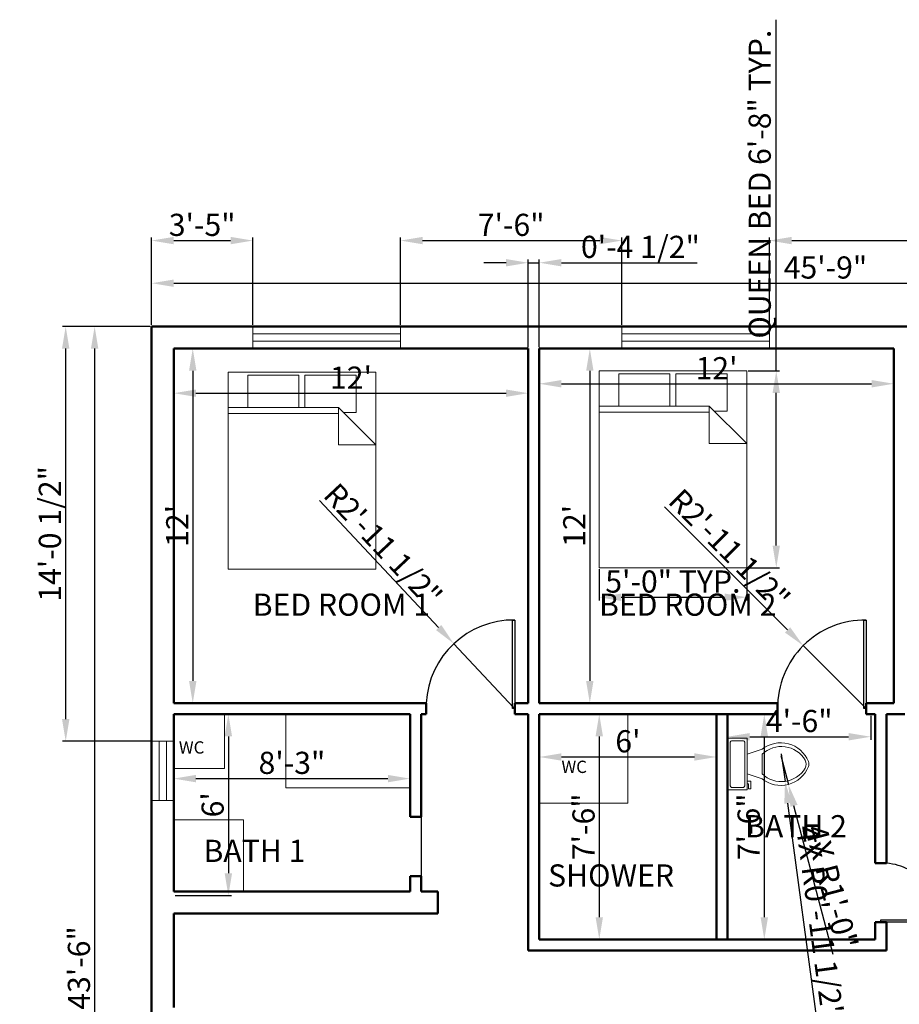
# Model space of a CAD drawing. Units: inches. Extents: x 145135 to 145817, y 90589 to 91373.
# Tile 3 of 4: x 145135 to 145493, y 90973 to 91373. Entities that reach past the tile are written whole.
import ezdxf

# ---------------------------------------------------------------- set-up
doc = ezdxf.new("R2010")
doc.units = ezdxf.units.IN
for name, color, linetype, lineweight in [('A-ANNO-DIMS', 2, 'Continuous', 18), ('A-ANNO-TEXT', 7, 'Continuous', 18), ('A-AREA-IDEN', 7, 'Continuous', 25), ('A-DOOR', 3, 'Continuous', 25), ('A-FLOR-FIXT', 9, 'Continuous', 18), ('A-FURN', 8, 'Continuous', 18), ('A-GLAZ', 4, 'Continuous', 18), ('A-WALL', 7, 'Continuous', 50)]:
    doc.layers.add(name, color=color, linetype=linetype, lineweight=lineweight)
doc.styles.get("Standard").update_dxf_attribs({"font": 'arial.ttf'})
doc.dimstyles.new('ISO-25', dxfattribs={"dimtxt": 9, "dimasz": 9, "dimexe": 1.25, "dimexo": 0.625, "dimtad": 1, "dimdec": 1, "dimrnd": 9, "dimlunit": 3, "dimtxsty": 'Standard', "dimcen": 2.5, "dimadec": 0, "dimazin": 0, "dimtfac": 1, "dimtdec": 1, "dimtmove": 0, "dimatfit": 3, "dimfxl": 1, "dimarcsym": 0})

# ---------------------------------------------------------------- blocks, each defined once
blk = doc.blocks.new('*D1')
at = {"layer": 'A-ANNO-DIMS', "color": 0, "lineweight": -2, "transparency": 16777216}
for p, q in [((145188.93, 91249.14), (145188.93, 91267.35)), ((145197.93, 91266.1), (145727.43, 91266.1)), ((145736.43, 91249.14), (145736.43, 91267.35))]:
    blk.add_line(p, q, dxfattribs=at)
at = {"layer": 'A-ANNO-DIMS', "color": 0, "transparency": 16777216}
for points in [[(145197.93, 91267.6), (145197.93, 91264.6), (145188.93, 91266.1)], [(145727.43, 91267.6), (145727.43, 91264.6), (145736.43, 91266.1)]]:
    blk.add_solid(points, dxfattribs=at)
at = {"layer": 'Defpoints', "color": 0, "transparency": 16777216}
for p in [(145736.43, 91266.1), (145188.93, 91248.52), (145736.43, 91248.52)]:
    blk.add_point(p, dxfattribs=at)
at = {"layer": 'A-ANNO-DIMS', "color": 0, "transparency": 16777216, "insert": (145462.68, 91271.32), "char_height": 9, "attachment_point": 5}
blk.add_mtext('45\'-9"', dxfattribs=at)
blk = doc.blocks.new('*D2')
at = {"layer": 'A-ANNO-DIMS', "color": 0, "lineweight": -2, "transparency": 16777216}
for p, q in [((145188.31, 91248.52), (145164.53, 91248.52)), ((145165.78, 91239.52), (145165.78, 90736.31)), ((145188.31, 90727.31), (145164.53, 90727.31))]:
    blk.add_line(p, q, dxfattribs=at)
at = {"layer": 'A-ANNO-DIMS', "color": 0, "transparency": 16777216}
for points in [[(145164.28, 91239.52), (145167.28, 91239.52), (145165.78, 91248.52)], [(145164.28, 90736.31), (145167.28, 90736.31), (145165.78, 90727.31)]]:
    blk.add_solid(points, dxfattribs=at)
at = {"layer": 'Defpoints', "color": 0, "transparency": 16777216}
for p in [(145188.93, 91248.52), (145165.78, 90727.31), (145188.93, 90727.31)]:
    blk.add_point(p, dxfattribs=at)
at = {"layer": 'A-ANNO-DIMS', "color": 0, "transparency": 16777216, "insert": (145160.56, 90987.92), "char_height": 9, "attachment_point": 5, "rotation": 90}
blk.add_mtext('43\'-6"', dxfattribs=at)
blk = doc.blocks.new('*D3')
at = {"layer": 'A-ANNO-DIMS', "color": 0, "lineweight": -2, "transparency": 16777216}
for p, q in [((145197.93, 91238.89), (145197.93, 91220.17)), ((145341.93, 91238.89), (145341.93, 91220.17)), ((145206.93, 91221.42), (145332.93, 91221.42))]:
    blk.add_line(p, q, dxfattribs=at)
at = {"layer": 'A-ANNO-DIMS', "color": 0, "transparency": 16777216}
for points in [[(145206.93, 91222.92), (145206.93, 91219.92), (145197.93, 91221.42)], [(145332.93, 91222.92), (145332.93, 91219.92), (145341.93, 91221.42)]]:
    blk.add_solid(points, dxfattribs=at)
at = {"layer": 'Defpoints', "color": 0, "transparency": 16777216}
for p in [(145197.93, 91239.52), (145341.93, 91239.52), (145341.93, 91221.42)]:
    blk.add_point(p, dxfattribs=at)
at = {"layer": 'A-ANNO-DIMS', "color": 0, "transparency": 16777216, "insert": (145269.93, 91226.57), "char_height": 9, "attachment_point": 5}
blk.add_mtext("12'", dxfattribs=at)
blk = doc.blocks.new('*D4')
at = {"layer": 'A-ANNO-DIMS', "color": 0, "lineweight": -2, "transparency": 16777216}
for p, q in [((145198.56, 91239.52), (145206.89, 91239.52)), ((145205.64, 91230.52), (145205.64, 91104.52)), ((145198.56, 91095.52), (145206.89, 91095.52))]:
    blk.add_line(p, q, dxfattribs=at)
at = {"layer": 'A-ANNO-DIMS', "color": 0, "transparency": 16777216}
for points in [[(145204.14, 91230.52), (145207.14, 91230.52), (145205.64, 91239.52)], [(145204.14, 91104.52), (145207.14, 91104.52), (145205.64, 91095.52)]]:
    blk.add_solid(points, dxfattribs=at)
at = {"layer": 'Defpoints', "color": 0, "transparency": 16777216}
for p in [(145197.93, 91239.52), (145197.93, 91095.52), (145205.64, 91095.52)]:
    blk.add_point(p, dxfattribs=at)
at = {"layer": 'A-ANNO-DIMS', "color": 0, "transparency": 16777216, "insert": (145200.5, 91167.52), "char_height": 9, "attachment_point": 5, "rotation": 90}
blk.add_mtext("12'", dxfattribs=at)
blk = doc.blocks.new('*D5')
at = {"layer": 'A-ANNO-DIMS', "color": 0, "lineweight": -2, "transparency": 16777216}
for p, q in [((145346.43, 91238.89), (145346.43, 91224.01)), ((145490.43, 91238.89), (145490.43, 91224.01)), ((145355.43, 91225.26), (145481.43, 91225.26))]:
    blk.add_line(p, q, dxfattribs=at)
at = {"layer": 'A-ANNO-DIMS', "color": 0, "transparency": 16777216}
for points in [[(145355.43, 91226.76), (145355.43, 91223.76), (145346.43, 91225.26)], [(145481.43, 91226.76), (145481.43, 91223.76), (145490.43, 91225.26)]]:
    blk.add_solid(points, dxfattribs=at)
at = {"layer": 'Defpoints', "color": 0, "transparency": 16777216}
for p in [(145346.43, 91239.52), (145490.43, 91239.52), (145490.43, 91225.26)]:
    blk.add_point(p, dxfattribs=at)
at = {"layer": 'A-ANNO-DIMS', "color": 0, "transparency": 16777216, "insert": (145418.43, 91230.41), "char_height": 9, "attachment_point": 5}
blk.add_mtext("12'", dxfattribs=at)
blk = doc.blocks.new('*D6')
at = {"layer": 'A-ANNO-DIMS', "color": 0, "lineweight": -2, "transparency": 16777216}
for p, q in [((145347.06, 91239.52), (145368.2, 91239.52)), ((145366.95, 91230.52), (145366.95, 91104.52)), ((145347.06, 91095.52), (145368.2, 91095.52))]:
    blk.add_line(p, q, dxfattribs=at)
at = {"layer": 'A-ANNO-DIMS', "color": 0, "transparency": 16777216}
for points in [[(145365.45, 91230.52), (145368.45, 91230.52), (145366.95, 91239.52)], [(145365.45, 91104.52), (145368.45, 91104.52), (145366.95, 91095.52)]]:
    blk.add_solid(points, dxfattribs=at)
at = {"layer": 'Defpoints', "color": 0, "transparency": 16777216}
for p in [(145346.43, 91239.52), (145346.43, 91095.52), (145366.95, 91095.52)]:
    blk.add_point(p, dxfattribs=at)
at = {"layer": 'A-ANNO-DIMS', "color": 0, "transparency": 16777216, "insert": (145361.8, 91167.52), "char_height": 9, "attachment_point": 5, "rotation": 90}
blk.add_mtext("12'", dxfattribs=at)
blk = doc.blocks.new('*D20')
at = {"layer": 'A-ANNO-DIMS', "color": 0, "lineweight": -2, "transparency": 16777216}
for p, q in [((145198.56, 91091.02), (145221.36, 91091.02)), ((145220.11, 91082.02), (145220.11, 91026.4)), ((145198.56, 91017.4), (145221.36, 91017.4))]:
    blk.add_line(p, q, dxfattribs=at)
at = {"layer": 'A-ANNO-DIMS', "color": 0, "transparency": 16777216}
for points in [[(145218.61, 91082.02), (145221.61, 91082.02), (145220.11, 91091.02)], [(145218.61, 91026.4), (145221.61, 91026.4), (145220.11, 91017.4)]]:
    blk.add_solid(points, dxfattribs=at)
at = {"layer": 'Defpoints', "color": 0, "transparency": 16777216}
for p in [(145197.93, 91091.02), (145197.93, 91017.4), (145220.11, 91017.4)]:
    blk.add_point(p, dxfattribs=at)
at = {"layer": 'A-ANNO-DIMS', "color": 0, "transparency": 16777216, "insert": (145214.89, 91054.21), "char_height": 9, "attachment_point": 5, "rotation": 90}
blk.add_mtext("6'", dxfattribs=at)
blk = doc.blocks.new('*D21')
at = {"layer": 'A-ANNO-DIMS', "color": 0, "lineweight": -2, "transparency": 16777216}
for p, q in [((145197.93, 91090.39), (145197.93, 91063.6)), ((145293.93, 91090.39), (145293.93, 91063.6)), ((145206.93, 91064.85), (145284.93, 91064.85))]:
    blk.add_line(p, q, dxfattribs=at)
at = {"layer": 'A-ANNO-DIMS', "color": 0, "transparency": 16777216}
for points in [[(145206.93, 91066.35), (145206.93, 91063.35), (145197.93, 91064.85)], [(145284.93, 91066.35), (145284.93, 91063.35), (145293.93, 91064.85)]]:
    blk.add_solid(points, dxfattribs=at)
at = {"layer": 'Defpoints', "color": 0, "transparency": 16777216}
for p in [(145197.93, 91091.02), (145293.93, 91091.02), (145293.93, 91064.85)]:
    blk.add_point(p, dxfattribs=at)
at = {"layer": 'A-ANNO-DIMS', "color": 0, "transparency": 16777216, "insert": (145245.93, 91070.08), "char_height": 9, "attachment_point": 5}
blk.add_mtext('8\'-3"', dxfattribs=at)
blk = doc.blocks.new('*D22')
at = {"layer": 'A-ANNO-DIMS', "color": 0, "lineweight": -2, "transparency": 16777216}
for p, q in [((145346.43, 91090.39), (145346.43, 91072.38)), ((145418.43, 91090.39), (145418.43, 91072.38)), ((145355.43, 91073.63), (145409.43, 91073.63))]:
    blk.add_line(p, q, dxfattribs=at)
at = {"layer": 'A-ANNO-DIMS', "color": 0, "transparency": 16777216}
for points in [[(145355.43, 91075.13), (145355.43, 91072.13), (145346.43, 91073.63)], [(145409.43, 91075.13), (145409.43, 91072.13), (145418.43, 91073.63)]]:
    blk.add_solid(points, dxfattribs=at)
at = {"layer": 'Defpoints', "color": 0, "transparency": 16777216}
for p in [(145346.43, 91091.02), (145418.43, 91091.02), (145418.43, 91073.63)]:
    blk.add_point(p, dxfattribs=at)
at = {"layer": 'A-ANNO-DIMS', "color": 0, "transparency": 16777216, "insert": (145382.43, 91078.85), "char_height": 9, "attachment_point": 5}
blk.add_mtext("6'", dxfattribs=at)
blk = doc.blocks.new('*D23')
at = {"layer": 'A-ANNO-DIMS', "color": 0, "lineweight": -2, "transparency": 16777216}
for p, q in [((145347.06, 91091.02), (145372.04, 91091.02)), ((145370.79, 91082.02), (145370.79, 91008.52)), ((145347.06, 90999.52), (145372.04, 90999.52))]:
    blk.add_line(p, q, dxfattribs=at)
at = {"layer": 'A-ANNO-DIMS', "color": 0, "transparency": 16777216}
for points in [[(145369.29, 91082.02), (145372.29, 91082.02), (145370.79, 91091.02)], [(145369.29, 91008.52), (145372.29, 91008.52), (145370.79, 90999.52)]]:
    blk.add_solid(points, dxfattribs=at)
at = {"layer": 'Defpoints', "color": 0, "transparency": 16777216}
for p in [(145346.43, 91091.02), (145346.43, 90999.52), (145370.79, 90999.52)]:
    blk.add_point(p, dxfattribs=at)
at = {"layer": 'A-ANNO-DIMS', "color": 0, "transparency": 16777216, "insert": (145365.57, 91045.27), "char_height": 9, "attachment_point": 5, "rotation": 90}
blk.add_mtext('7\'-6"', dxfattribs=at)
blk = doc.blocks.new('*D24')
at = {"layer": 'A-ANNO-DIMS', "color": 0, "lineweight": -2, "transparency": 16777216}
for p, q in [((145423.56, 91091.02), (145439.09, 91091.02)), ((145437.84, 91082.02), (145437.84, 91008.52)), ((145423.56, 90999.52), (145439.09, 90999.52))]:
    blk.add_line(p, q, dxfattribs=at)
at = {"layer": 'A-ANNO-DIMS', "color": 0, "transparency": 16777216}
for points in [[(145436.34, 91082.02), (145439.34, 91082.02), (145437.84, 91091.02)], [(145436.34, 91008.52), (145439.34, 91008.52), (145437.84, 90999.52)]]:
    blk.add_solid(points, dxfattribs=at)
at = {"layer": 'Defpoints', "color": 0, "transparency": 16777216}
for p in [(145422.93, 91091.02), (145422.93, 90999.52), (145437.84, 90999.52)]:
    blk.add_point(p, dxfattribs=at)
at = {"layer": 'A-ANNO-DIMS', "color": 0, "transparency": 16777216, "insert": (145432.62, 91045.27), "char_height": 9, "attachment_point": 5, "rotation": 90}
blk.add_mtext('7\'-6"', dxfattribs=at)
blk = doc.blocks.new('*D25')
at = {"layer": 'A-ANNO-DIMS', "color": 0, "lineweight": -2, "transparency": 16777216}
for p, q in [((145422.93, 91090.39), (145422.93, 91080.6)), ((145481.1, 91090.39), (145481.1, 91080.6)), ((145431.93, 91081.85), (145472.1, 91081.85))]:
    blk.add_line(p, q, dxfattribs=at)
at = {"layer": 'A-ANNO-DIMS', "color": 0, "transparency": 16777216}
for points in [[(145431.93, 91083.35), (145431.93, 91080.35), (145422.93, 91081.85)], [(145472.1, 91083.35), (145472.1, 91080.35), (145481.1, 91081.85)]]:
    blk.add_solid(points, dxfattribs=at)
at = {"layer": 'Defpoints', "color": 0, "transparency": 16777216}
for p in [(145422.93, 91091.02), (145481.1, 91091.02), (145481.1, 91081.85)]:
    blk.add_point(p, dxfattribs=at)
at = {"layer": 'A-ANNO-DIMS', "color": 0, "transparency": 16777216, "insert": (145452.02, 91087.07), "char_height": 9, "attachment_point": 5}
blk.add_mtext('4\'-6"', dxfattribs=at)
blk = doc.blocks.new('Toilet - top')
for p, q in [((9.5, -6), (9.5, -2)), ((-8, -8.5), (-8, -8)), ((-7, -8), (-7, -9.5)), ((-4, -8), (-6, -14)), ((4, -8), (6, -14)), ((-10, -8.5), (-8, -8.5)), ((-10, -9.5), (-10, -8.5)), ((-7, -9.5), (-10, -9.5)), ((4, -14), (-4, -14))]:
    blk.add_line(p, q)
blk.add_lwpolyline([(10.5, -8), (10.5, 0), (-10.5, 0), (-10.5, -8)], close=True)
for points in [[(-9.5, -2), (-9.5, -6)], [(8.5, -1), (-8.5, -1)], [(-8.5, -7), (8.5, -7)]]:
    blk.add_lwpolyline(points)
for centre, radius, start, end in [((-8.62, -1.88), 0.884, 81.8699, 188.1301), ((8.62, -1.88), 0.884, 351.8699, 98.1301), ((-8.62, -6.12), 0.884, 171.8699, 278.1301), ((8.62, -6.12), 0.884, 261.8699, 8.1301), ((3.52, -21.58), 12.17, 141.4691, 247.9714), ((4.2, -21.82), 11.33, 136.3677, 238.9468), ((-3.52, -21.58), 12.17, 292.0284, 38.5307), ((-4.2, -21.82), 11.33, 301.053, 43.6321), ((0, -27.88), 4, 245.7318, 294.2682), ((0, -29), 4, 254.8605, 285.1395)]:
    blk.add_arc(centre, radius, start, end)
blk = doc.blocks.new('Bed - Queen')
for p, q in [((0, -80.00003), (0, 0)), ((0, 0), (59.99999, 0)), ((59.99999, 0), (59.99999, -80.00003)), ((7.99999, -1.2), (28.79998, -1.2)), ((7.99999, -14.4), (7.99999, -1.2)), ((28.79998, -1.2), (28.79998, -14.4)), ((31.19999, -1.2), (51.99999, -1.2)), ((31.19999, -14.4), (31.19999, -1.2)), ((51.99999, -1.2), (51.99999, -16.4)), ((0, -14.4), (44.8, -14.4)), ((59.99999, -29.6), (44.8, -14.4)), ((44.8, -14.4), (44.8, -29.6)), ((44.8, -16.8), (0, -16.8)), ((51.99999, -16.4), (46.79936, -16.4)), ((44.8, -29.6), (59.99999, -29.6)), ((59.99999, -80.00003), (0, -80.00003))]:
    blk.add_line(p, q)
blk = doc.blocks.new('WIN-60IN')
for p, q in [((0, 9), (0, 0)), ((60, 9), (60, 0)), ((60, 6), (0, 6)), ((60, 3), (0, 3))]:
    blk.add_line(p, q)
blk = doc.blocks.new('WIN-24IN')
for p, q in [((0, 24), (9, 24)), ((3, 0), (3, 24)), ((6, 0), (6, 24)), ((0, 0), (9, 0))]:
    blk.add_line(p, q)
blk = doc.blocks.new('*D40')
at = {"layer": 'A-ANNO-DIMS', "color": 0, "lineweight": -2, "transparency": 16777216}
for p, q in [((145442.7, 91230.52), (145442.7, 91373.16)), ((145431.32, 91230.52), (145443.95, 91230.52)), ((145442.7, 91159.52), (145442.7, 91221.52)), ((145431.32, 91150.52), (145443.95, 91150.52))]:
    blk.add_line(p, q, dxfattribs=at)
at = {"layer": 'A-ANNO-DIMS', "color": 0, "transparency": 16777216}
for points in [[(145441.2, 91221.52), (145444.2, 91221.52), (145442.7, 91230.52)], [(145441.2, 91159.52), (145444.2, 91159.52), (145442.7, 91150.52)]]:
    blk.add_solid(points, dxfattribs=at)
at = {"layer": 'Defpoints', "color": 0, "transparency": 16777216}
for p in [(145430.7, 91230.52), (145442.7, 91230.52), (145430.7, 91150.52)]:
    blk.add_point(p, dxfattribs=at)
at = {"layer": 'A-ANNO-DIMS', "color": 0, "transparency": 16777216, "insert": (145437.14, 91306.34), "char_height": 9, "attachment_point": 5, "rotation": 90}
blk.add_mtext('QUEEN BED 6\'-8" TYP.', dxfattribs=at)
blk = doc.blocks.new('*D41')
at = {"layer": 'A-ANNO-DIMS', "color": 0, "lineweight": -2, "transparency": 16777216}
for p, q in [((145370.7, 91149.89), (145370.7, 91137.27)), ((145430.7, 91149.89), (145430.7, 91137.27)), ((145379.7, 91138.52), (145421.7, 91138.52))]:
    blk.add_line(p, q, dxfattribs=at)
at = {"layer": 'A-ANNO-DIMS', "color": 0, "transparency": 16777216}
for points in [[(145379.7, 91140.02), (145379.7, 91137.02), (145370.7, 91138.52)], [(145421.7, 91140.02), (145421.7, 91137.02), (145430.7, 91138.52)]]:
    blk.add_solid(points, dxfattribs=at)
at = {"layer": 'Defpoints', "color": 0, "transparency": 16777216}
for p in [(145370.7, 91150.52), (145430.7, 91150.52), (145430.7, 91138.52)]:
    blk.add_point(p, dxfattribs=at)
at = {"layer": 'A-ANNO-DIMS', "color": 0, "transparency": 16777216, "insert": (145400.7, 91143.74), "char_height": 9, "attachment_point": 5}
blk.add_mtext('5\'-0" TYP.', dxfattribs=at)
blk = doc.blocks.new('*D57')
at = {"layer": 'A-ANNO-DIMS', "color": 0, "lineweight": -2, "transparency": 16777216}
for p, q in [((145188.93, 91249.14), (145188.93, 91284.67)), ((145230, 91249.14), (145230, 91284.67)), ((145197.93, 91283.42), (145221, 91283.42))]:
    blk.add_line(p, q, dxfattribs=at)
at = {"layer": 'A-ANNO-DIMS', "color": 0, "transparency": 16777216}
for points in [[(145197.93, 91284.92), (145197.93, 91281.92), (145188.93, 91283.42)], [(145221, 91284.92), (145221, 91281.92), (145230, 91283.42)]]:
    blk.add_solid(points, dxfattribs=at)
at = {"layer": 'Defpoints', "color": 0, "transparency": 16777216}
for p in [(145230, 91283.42), (145188.93, 91248.52), (145230, 91248.52)]:
    blk.add_point(p, dxfattribs=at)
at = {"layer": 'A-ANNO-DIMS', "color": 0, "transparency": 16777216, "insert": (145209.47, 91288.64), "char_height": 9, "attachment_point": 5}
blk.add_mtext('3\'-5"', dxfattribs=at)
blk = doc.blocks.new('*D58')
at = {"layer": 'A-ANNO-DIMS', "color": 0, "lineweight": -2, "transparency": 16777216}
for p, q in [((145290, 91249.14), (145290, 91284.67)), ((145380, 91249.14), (145380, 91284.67)), ((145299, 91283.42), (145371, 91283.42))]:
    blk.add_line(p, q, dxfattribs=at)
at = {"layer": 'A-ANNO-DIMS', "color": 0, "transparency": 16777216}
for points in [[(145299, 91284.92), (145299, 91281.92), (145290, 91283.42)], [(145371, 91284.92), (145371, 91281.92), (145380, 91283.42)]]:
    blk.add_solid(points, dxfattribs=at)
at = {"layer": 'Defpoints', "color": 0, "transparency": 16777216}
for p in [(145380, 91283.42), (145290, 91248.52), (145380, 91248.52)]:
    blk.add_point(p, dxfattribs=at)
at = {"layer": 'A-ANNO-DIMS', "color": 0, "transparency": 16777216, "insert": (145335, 91288.64), "char_height": 9, "attachment_point": 5}
blk.add_mtext('7\'-6"', dxfattribs=at)
blk = doc.blocks.new('*D59')
at = {"layer": 'A-ANNO-DIMS', "color": 0, "lineweight": -2, "transparency": 16777216}
for p, q in [((145440, 91249.14), (145440, 91284.67)), ((145640, 91249.14), (145640, 91284.67)), ((145449, 91283.42), (145631, 91283.42))]:
    blk.add_line(p, q, dxfattribs=at)
at = {"layer": 'A-ANNO-DIMS', "color": 0, "transparency": 16777216}
for points in [[(145449, 91284.92), (145449, 91281.92), (145440, 91283.42)], [(145631, 91284.92), (145631, 91281.92), (145640, 91283.42)]]:
    blk.add_solid(points, dxfattribs=at)
at = {"layer": 'Defpoints', "color": 0, "transparency": 16777216}
for p in [(145640, 91283.42), (145440, 91248.52), (145640, 91248.52)]:
    blk.add_point(p, dxfattribs=at)
at = {"layer": 'A-ANNO-DIMS', "color": 0, "transparency": 16777216, "insert": (145540, 91288.64), "char_height": 9, "attachment_point": 5}
blk.add_mtext('16\'-8"', dxfattribs=at)
blk = doc.blocks.new('*D64')
at = {"layer": 'A-ANNO-DIMS', "color": 0, "lineweight": -2, "transparency": 16777216}
for p, q in [((145188.31, 91248.52), (145152.78, 91248.52)), ((145154.03, 91089), (145154.03, 91239.52)), ((145188.31, 91080), (145152.78, 91080))]:
    blk.add_line(p, q, dxfattribs=at)
at = {"layer": 'A-ANNO-DIMS', "color": 0, "transparency": 16777216}
for points in [[(145152.53, 91239.52), (145155.53, 91239.52), (145154.03, 91248.52)], [(145152.53, 91089), (145155.53, 91089), (145154.03, 91080)]]:
    blk.add_solid(points, dxfattribs=at)
at = {"layer": 'Defpoints', "color": 0, "transparency": 16777216}
for p in [(145154.03, 91248.52), (145188.93, 91248.52), (145188.93, 91080)]:
    blk.add_point(p, dxfattribs=at)
at = {"layer": 'A-ANNO-DIMS', "color": 0, "transparency": 16777216, "insert": (145148.76, 91164.26), "char_height": 9, "attachment_point": 5, "rotation": 90}
blk.add_mtext('14\'-0 1/2"', dxfattribs=at)
blk = doc.blocks.new('*D67')
at = {"layer": 'A-ANNO-DIMS', "color": 0, "lineweight": -2, "transparency": 16777216}
for p, q in [((145332.93, 91274.42), (145323.93, 91274.42)), ((145341.93, 91240.14), (145341.93, 91275.67)), ((145341.93, 91274.42), (145346.43, 91274.42)), ((145346.43, 91240.14), (145346.43, 91275.67)), ((145355.43, 91274.42), (145410.58, 91274.42))]:
    blk.add_line(p, q, dxfattribs=at)
at = {"layer": 'A-ANNO-DIMS', "color": 0, "transparency": 16777216}
for points in [[(145332.93, 91275.92), (145332.93, 91272.92), (145341.93, 91274.42)], [(145355.43, 91275.92), (145355.43, 91272.92), (145346.43, 91274.42)]]:
    blk.add_solid(points, dxfattribs=at)
at = {"layer": 'Defpoints', "color": 0, "transparency": 16777216}
for p in [(145346.43, 91274.42), (145341.93, 91239.52), (145346.43, 91239.52)]:
    blk.add_point(p, dxfattribs=at)
at = {"layer": 'A-ANNO-DIMS', "color": 0, "transparency": 16777216, "insert": (145387.51, 91279.7), "char_height": 9, "attachment_point": 5}
blk.add_mtext('0\'-4 1/2"', dxfattribs=at)
blk = doc.blocks.new('*D76')
at = {"layer": 'A-ANNO-DIMS', "color": 0, "lineweight": -2, "transparency": 16777216}
for p, q in [((145257.15, 91177.84), (145305.54, 91126.22)), ((145336.01, 91093.73), (145311.7, 91119.66))]:
    blk.add_line(p, q, dxfattribs=at)
at = {"layer": 'A-ANNO-DIMS', "color": 0, "transparency": 16777216}
blk.add_solid([(145306.64, 91127.25), (145304.45, 91125.2), (145311.7, 91119.66)], dxfattribs=at)
at = {"layer": 'Defpoints', "color": 0, "transparency": 16777216}
for p in [(145311.7, 91119.66), (145336.01, 91093.73)]:
    blk.add_point(p, dxfattribs=at)
at = {"layer": 'A-ANNO-DIMS', "color": 0, "transparency": 16777216, "insert": (145282.12, 91158.92), "char_height": 9, "attachment_point": 5, "rotation": 313.1529}
blk.add_mtext('R2\'-11 1/2"', dxfattribs=at)
blk = doc.blocks.new('*D77')
at = {"layer": 'A-ANNO-DIMS', "color": 0, "lineweight": -2, "transparency": 16777216}
for p, q in [((145397.27, 91175.26), (145447.3, 91125.24)), ((145478.76, 91093.77), (145453.66, 91118.87))]:
    blk.add_line(p, q, dxfattribs=at)
at = {"layer": 'A-ANNO-DIMS', "color": 0, "transparency": 16777216}
blk.add_solid([(145448.36, 91126.3), (145446.23, 91124.18), (145453.66, 91118.87)], dxfattribs=at)
at = {"layer": 'Defpoints', "color": 0, "transparency": 16777216}
for p in [(145453.66, 91118.87), (145478.76, 91093.77)]:
    blk.add_point(p, dxfattribs=at)
at = {"layer": 'A-ANNO-DIMS', "color": 0, "transparency": 16777216, "insert": (145422.83, 91157.16), "char_height": 9, "attachment_point": 5, "rotation": 315.0007}
blk.add_mtext('R2\'-11 1/2"', dxfattribs=at)
blk = doc.blocks.new('*D83')
at = {"layer": 'A-ANNO-DIMS', "color": 0, "lineweight": -2, "transparency": 16777216}
for p, q in [((145444.52, 91074.27), (145447.61, 91062.5)), ((145465.77, 90993.36), (145449.89, 91053.8))]:
    blk.add_line(p, q, dxfattribs=at)
at = {"layer": 'A-ANNO-DIMS', "color": 0, "transparency": 16777216}
blk.add_solid([(145451.34, 91054.18), (145448.44, 91053.42), (145447.61, 91062.5)], dxfattribs=at)
at = {"layer": 'Defpoints', "color": 0, "transparency": 16777216}
for p in [(145444.52, 91074.27), (145447.61, 91062.5)]:
    blk.add_point(p, dxfattribs=at)
at = {"layer": 'A-ANNO-DIMS', "color": 0, "transparency": 16777216, "insert": (145464.03, 91020.56), "char_height": 9, "attachment_point": 5, "rotation": 284.7198}
blk.add_mtext('4X R1\'-0"', dxfattribs=at)
blk = doc.blocks.new('*D84')
at = {"layer": 'A-ANNO-DIMS', "color": 0, "lineweight": -2, "transparency": 16777216}
for p, q in [((145444.75, 91074.95), (145446.26, 91063.73)), ((145459.51, 90965.16), (145447.46, 91054.81))]:
    blk.add_line(p, q, dxfattribs=at)
at = {"layer": 'A-ANNO-DIMS', "color": 0, "transparency": 16777216}
blk.add_solid([(145448.95, 91055.01), (145445.97, 91054.61), (145446.26, 91063.73)], dxfattribs=at)
at = {"layer": 'Defpoints', "color": 0, "transparency": 16777216}
for p in [(145444.75, 91074.95), (145446.26, 91063.73)]:
    blk.add_point(p, dxfattribs=at)
at = {"layer": 'A-ANNO-DIMS', "color": 0, "transparency": 16777216, "insert": (145459.32, 91006.23), "char_height": 9, "attachment_point": 5, "rotation": 277.655}
blk.add_mtext('4X R0\'-11 1/2"', dxfattribs=at)

msp = doc.modelspace()

# ---------------------------------------------------------------- linework, layer by layer
at = {"layer": 'A-DOOR'}
for p, q in [((145335.51, 91093.27), (145335.51, 91129.27)), ((145335.51, 91129.27), (145336.51, 91129.27)), ((145336.51, 91129.27), (145336.51, 91095.52)), ((145478.26, 91093.27), (145478.26, 91129.27)), ((145478.26, 91129.27), (145479.26, 91129.27)), ((145479.26, 91129.27), (145479.26, 91095.52)), ((145336.51, 91093.27), (145335.51, 91093.27)), ((145479.26, 91093.27), (145478.26, 91093.27)), ((145298.43, 91049.27), (145298.43, 91025.27)), ((145485.18, 91006.53), (145485.18, 91007.53)), ((145485.18, 91007.53), (145509.18, 91007.53)), ((145509.18, 91006.53), (145487.43, 91006.53))]:
    msp.add_line(p, q, dxfattribs=at)
for centre, radius, start, end in [((145336.01, 91093.73), 35.55, 89.194, 177.1108), ((145478.76, 91093.77), 35.5, 89.1931, 180.8069), ((145485.68, 91007.03), 23.51, 358.7811, 91.2189)]:
    msp.add_arc(centre, radius, start, end, dxfattribs=at)
at = {"layer": 'A-FLOR-FIXT'}
for p, q in [((145218.6, 91091.02), (145218.6, 91069)), ((145243.5, 91091.02), (145243.5, 91061.12)), ((145382.43, 91091.02), (145382.43, 91054.88)), ((145218.6, 91069), (145197.93, 91069)), ((145243.5, 91061.12), (145293.93, 91061.12)), ((145382.43, 91054.88), (145346.43, 91054.88)), ((145197.93, 91048.09), (145226.3, 91048.09)), ((145226.3, 91048.09), (145226.3, 91019.02))]:
    msp.add_line(p, q, dxfattribs=at)
at = {"layer": 'A-WALL'}
for p, q in [((145736.43, 91248.52), (145188.93, 91248.52)), ((145188.93, 90727.31), (145188.93, 91248.52)), ((145341.93, 91239.52), (145197.93, 91239.52)), ((145197.93, 91095.52), (145197.93, 91239.52)), ((145341.93, 91095.52), (145341.93, 91239.52)), ((145346.43, 91095.52), (145346.43, 91239.52)), ((145490.43, 91239.52), (145346.43, 91239.52)), ((145490.43, 91095.52), (145490.43, 91239.52)), ((145300.51, 91095.52), (145197.93, 91095.52)), ((145300.51, 91095.52), (145300.51, 91091.02)), ((145341.93, 91095.52), (145336.51, 91095.52)), ((145336.51, 91095.52), (145336.51, 91091.02)), ((145443.26, 91095.52), (145346.43, 91095.52)), ((145443.26, 91095.52), (145443.26, 91091.02)), ((145490.43, 91095.52), (145479.26, 91095.52)), ((145479.26, 91095.52), (145479.26, 91091.02)), ((145197.93, 91019.02), (145197.93, 91091.02)), ((145293.93, 91091.02), (145197.93, 91091.02)), ((145293.93, 91049.27), (145293.93, 91091.02)), ((145298.43, 91049.27), (145298.43, 91091.02)), ((145300.51, 91091.02), (145298.43, 91091.02)), ((145341.93, 91091.02), (145336.51, 91091.02)), ((145341.93, 91091.02), (145341.93, 90995.02)), ((145418.43, 91091.02), (145346.43, 91091.02)), ((145346.43, 91019.02), (145346.43, 91091.02)), ((145443.26, 91091.02), (145346.43, 91091.02)), ((145418.43, 90999.52), (145418.43, 91091.02)), ((145422.93, 90999.52), (145422.93, 91091.02)), ((145482.93, 91091.02), (145479.26, 91091.02)), ((145482.93, 91030.53), (145482.93, 91091.02)), ((145494.93, 91091.02), (145487.43, 91091.02)), ((145487.43, 91030.53), (145487.43, 91091.02)), ((145494.93, 91091.02), (145490.43, 91091.02)), ((145293.93, 91049.27), (145298.43, 91049.27)), ((145482.93, 91030.53), (145487.43, 91030.53)), ((145293.93, 91019.02), (145293.93, 91025.27)), ((145293.93, 91025.27), (145298.43, 91025.27)), ((145298.43, 91019.02), (145298.43, 91025.27)), ((145293.93, 91019.02), (145197.93, 91019.02)), ((145305.26, 91019.02), (145298.43, 91019.02)), ((145305.26, 91019.02), (145305.26, 91010.02)), ((145346.43, 91010.02), (145346.43, 91019.02)), ((145305.26, 91010.02), (145197.93, 91010.02)), ((145197.93, 90971.81), (145197.93, 91010.02)), ((145341.93, 90995.02), (145341.93, 91010.02)), ((145346.43, 90999.52), (145346.43, 91010.02)), ((145482.93, 90999.52), (145482.93, 91006.53)), ((145482.93, 91006.53), (145487.43, 91006.53)), ((145487.43, 90995.02), (145487.43, 91006.53)), ((145482.93, 90999.52), (145346.43, 90999.52)), ((145487.43, 90995.02), (145341.93, 90995.02))]:
    msp.add_line(p, q, dxfattribs=at)

# ---------------------------------------------------------------- block references
at = {"layer": 'A-FLOR-FIXT', "rotation": 89.99999999999999}
msp.add_blockref('Toilet - top', (145422.93, 91070.75), dxfattribs=at)
at = {"layer": 'A-FURN'}
for p in [(145220, 91230), (145370.7, 91230.52)]:
    msp.add_blockref('Bed - Queen', p, dxfattribs=at)
at = {"layer": 'A-GLAZ'}
for name, p in [('WIN-60IN', (145230, 91239.52)), ('WIN-60IN', (145380, 91239.52)), ('WIN-24IN', (145188.93, 91056))]:
    msp.add_blockref(name, p, dxfattribs=at)

# ---------------------------------------------------------------- texts
at = {"layer": 'A-ANNO-TEXT', "char_height": 5, "attachment_point": 1}
for insert in [(145200, 91080), (145355.43, 91072.13)]:
    msp.add_mtext_dynamic_manual_height_columns('WC ', width=20.1144, gutter_width=12.5, heights=[0], dxfattribs=dict(at, insert=insert))
at = {"layer": 'A-AREA-IDEN', "char_height": 9, "attachment_point": 1}
for s, insert in [('BED ROOM 1', (145230, 91140)), ('BED ROOM 2', (145370.7, 91140)), ('BATH 2', (145430, 91050)), ('BATH 1', (145210, 91040)), ('SHOWER', (145350, 91030))]:
    msp.add_mtext_dynamic_manual_height_columns(s, width=90, gutter_width=12.5, heights=[0], dxfattribs=dict(at, insert=insert))

# ---------------------------------------------------------------- dimensions: what is measured, and where the dimension line sits
at = {"layer": 'A-ANNO-DIMS'}
dim = msp.add_linear_dim(base=(145442.7, 91230.52), p1=(145430.7, 91150.52), p2=(145430.7, 91230.52), angle=90, text='QUEEN BED <> TYP.', dimstyle='ISO-25', override={"dimdec": 1, "dimlfac": 1, "dimrnd": 0, "dimzin": 1, "dimdsep": 46, "dimlunit": 4, "dimfrac": 2}, dxfattribs=at)
dim.commit()
dim.dimension.update_dxf_attribs({"geometry": '*D40', "text_midpoint": (145437.14, 91306.34)})
for base, p1, p2, override, picture, middle in [((145230, 91283.42), (145188.93, 91248.52), (145230, 91248.52), {"dimdec": 1, "dimlfac": 1, "dimrnd": 0, "dimzin": 1, "dimdsep": 46, "dimlunit": 4, "dimfrac": 2}, '*D57', (145209.47, 91288.64)), ((145380, 91283.42), (145290, 91248.52), (145380, 91248.52), {"dimdec": 1, "dimlfac": 1, "dimrnd": 0, "dimzin": 1, "dimdsep": 46, "dimlunit": 4, "dimfrac": 2}, '*D58', (145335, 91288.64)), ((145346.43, 91274.42), (145341.93, 91239.52), (145346.43, 91239.52), {"dimdec": 1, "dimlfac": 1, "dimrnd": 0, "dimzin": 1, "dimdsep": 46, "dimlunit": 4, "dimfrac": 2}, '*D67', (145387.51, 91279.7)), ((145640, 91283.42), (145440, 91248.52), (145640, 91248.52), {"dimdec": 1, "dimlfac": 1, "dimrnd": 0, "dimzin": 1, "dimdsep": 46, "dimlunit": 4, "dimfrac": 2}, '*D59', (145540, 91288.64)), ((145736.43, 91266.1), (145188.93, 91248.52), (145736.43, 91248.52), {"dimclrd": 0, "dimclre": 0, "dimclrt": 0}, '*D1', (145462.68, 91271.32)), ((145341.93, 91221.42), (145197.93, 91239.52), (145341.93, 91239.52), {"dimclrd": 0, "dimclre": 0, "dimclrt": 0}, '*D3', (145269.93, 91226.57)), ((145490.43, 91225.26), (145346.43, 91239.52), (145490.43, 91239.52), {"dimclrd": 0, "dimclre": 0, "dimclrt": 0}, '*D5', (145418.43, 91230.41)), ((145481.1, 91081.85), (145422.93, 91091.02), (145481.1, 91091.02), {"dimclrd": 0, "dimclre": 0, "dimclrt": 0}, '*D25', (145452.02, 91087.07)), ((145293.93, 91064.85), (145197.93, 91091.02), (145293.93, 91091.02), {"dimclrd": 0, "dimclre": 0, "dimclrt": 0}, '*D21', (145245.93, 91070.08)), ((145418.43, 91073.63), (145346.43, 91091.02), (145418.43, 91091.02), {"dimclrd": 0, "dimclre": 0, "dimclrt": 0}, '*D22', (145382.43, 91078.85))]:
    dim = msp.add_linear_dim(base=base, p1=p1, p2=p2, dimstyle='ISO-25', override=override, dxfattribs=at)
    dim.commit()
    dim.dimension.update_dxf_attribs({"geometry": picture, "text_midpoint": middle})
for base, p1, p2, override, picture, middle in [((145154.03, 91248.52), (145188.93, 91080), (145188.93, 91248.52), {"dimdec": 1, "dimlfac": 1, "dimrnd": 0, "dimzin": 1, "dimdsep": 46, "dimlunit": 4, "dimfrac": 2}, '*D64', (145148.76, 91164.26)), ((145165.78, 90727.31), (145188.93, 91248.52), (145188.93, 90727.31), {"dimclrd": 0, "dimclre": 0, "dimclrt": 0}, '*D2', (145160.56, 90987.92)), ((145205.64, 91095.52), (145197.93, 91239.52), (145197.93, 91095.52), {"dimclrd": 0, "dimclre": 0, "dimclrt": 0}, '*D4', (145200.5, 91167.52)), ((145366.95, 91095.52), (145346.43, 91239.52), (145346.43, 91095.52), {"dimclrd": 0, "dimclre": 0, "dimclrt": 0}, '*D6', (145361.8, 91167.52)), ((145220.11, 91017.4), (145197.93, 91091.02), (145197.93, 91017.4), {"dimclrd": 0, "dimclre": 0, "dimclrt": 0}, '*D20', (145214.89, 91054.21)), ((145370.79, 90999.52), (145346.43, 91091.02), (145346.43, 90999.52), {"dimclrd": 0, "dimclre": 0, "dimclrt": 0}, '*D23', (145365.57, 91045.27)), ((145437.84, 90999.52), (145422.93, 91091.02), (145422.93, 90999.52), {"dimclrd": 0, "dimclre": 0, "dimclrt": 0}, '*D24', (145432.62, 91045.27))]:
    dim = msp.add_linear_dim(base=base, p1=p1, p2=p2, angle=90, dimstyle='ISO-25', override=override, dxfattribs=at)
    dim.commit()
    dim.dimension.update_dxf_attribs({"geometry": picture, "text_midpoint": middle})
for center, mpoint, picture, middle in [((145336.01, 91093.73), (145311.7, 91119.66), '*D76', (145282.12, 91158.92)), ((145478.76, 91093.77), (145453.66, 91118.87), '*D77', (145422.83, 91157.16))]:
    dim = msp.add_radius_dim(center=center, mpoint=mpoint, dimstyle='ISO-25', override={"dimdec": 1, "dimlfac": 1, "dimrnd": 0, "dimzin": 1, "dimdsep": 46, "dimlunit": 4, "dimfrac": 2}, dxfattribs=at)
    dim.commit()
    dim.dimension.update_dxf_attribs({"geometry": picture, "text_midpoint": middle})
dim = msp.add_linear_dim(base=(145430.7, 91138.52), p1=(145370.7, 91150.52), p2=(145430.7, 91150.52), text='<> TYP.', dimstyle='ISO-25', override={"dimdec": 1, "dimlfac": 1, "dimrnd": 0, "dimzin": 1, "dimdsep": 46, "dimlunit": 4, "dimfrac": 2}, dxfattribs=at)
dim.commit()
dim.dimension.update_dxf_attribs({"geometry": '*D41', "text_midpoint": (145400.7, 91143.74)})
for center, mpoint, picture, middle in [((145444.75, 91074.95), (145446.26, 91063.73), '*D84', (145459.32, 91006.23)), ((145444.52, 91074.27), (145447.61, 91062.5), '*D83', (145464.03, 91020.56))]:
    dim = msp.add_radius_dim(center=center, mpoint=mpoint, text='4X <>', dimstyle='ISO-25', override={"dimdec": 1, "dimlfac": 1, "dimrnd": 0, "dimzin": 1, "dimdsep": 46, "dimlunit": 4, "dimfrac": 2}, dxfattribs=at)
    dim.commit()
    dim.dimension.update_dxf_attribs({"geometry": picture, "text_midpoint": middle})

doc.saveas('drawing.dxf')
